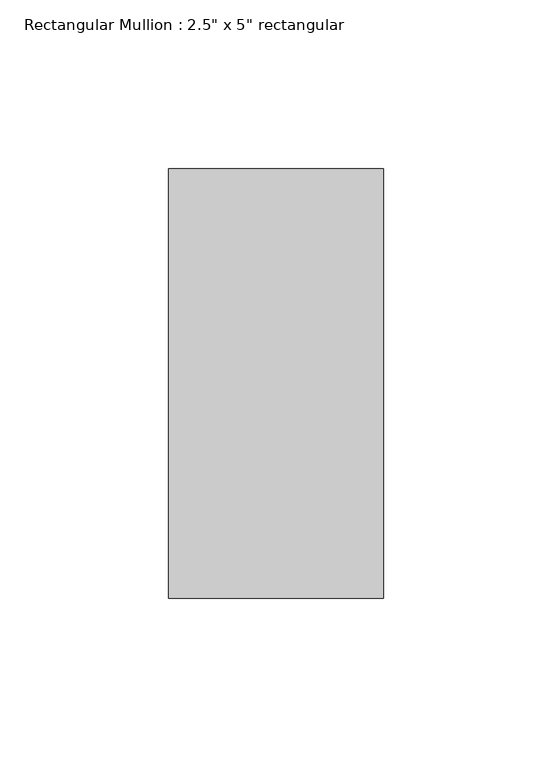
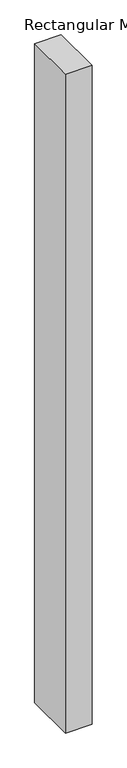
"""IFC4 building model written with IfcOpenShell, lengths in millimetres: member geometry."""

from ifc_helpers import new_model, si_unit, frame, origin, place, context, project, spatial, polyline, outline, extrude, source, transform, mapped, element, save


def member_cfa26838(model_context):
    return source(origin(), model_context, "Body", "SweptSolid", [
        extrude(outline(polyline([(31.75, 63.5), (31.75, -63.5), (-31.75, -63.5), (-31.75, 63.5), (31.75, 63.5)])), frame((0.0, 0.0, -1665.799372), z_axis=(0.0, 0.0, 1.0), x_axis=(1.0, 0.0, 0.0)), (0.0, 0.0, 1.0), 1665.799372),
    ])


if __name__ == "__main__":
    model = new_model("IFC4")
    model_context = context("Model", 3, world=origin())
    ifc_project = project(units=[si_unit("LENGTHUNIT", "METRE", prefix="MILLI")], contexts=[model_context])
    site = spatial("IfcSite", under=ifc_project)
    building = spatial("IfcBuilding", under=site)
    placement = place(None, origin())
    member_shape = member_cfa26838(model_context)
    element("IfcMember", 1, ObjectType="Rectangular Mullion : 2.5\" x 5\" rectangular", at=placement, inside=building, context=model_context, shape_type="MappedRepresentation", body=[
        mapped(member_shape, transform((0.0, 0.0, 0.0), x_axis=(1.0, 0.0, 0.0), y_axis=(0.0, 1.0, 0.0), z_axis=(0.0, 0.0, 1.0))),
    ])
    save(model, "model.ifc")

# Revit data of these elements
# Type "Rectangular Mullion : 2.5\" x 5\" rectangular"
#   built-in parameter 1007304 = 0.416667 (stored number, unit not read)
#   built-in parameter 1007301 = 0.104167 (stored number, unit not read)
#   built-in parameter 1007300 = 0.104167 (stored number, unit not read)
# Element 1 (IfcMember, "Rectangular Mullion : 2.5\" x 5\" rectangular")
#   Materials on its faces: "Aluminum"
# Materials
#   "Aluminum": class "Metal", colour RGB 247 247 247, transparency 0, Description = "Aluminum 6061", Cost = 0
